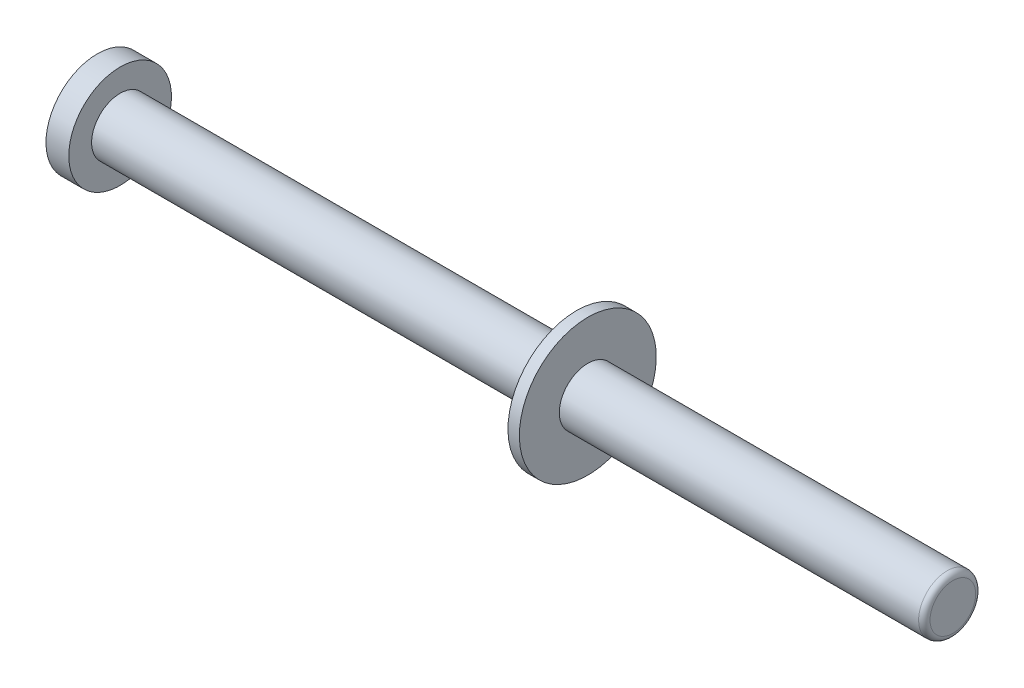
SolidWorks part; units mm, degrees
material "Plain Carbon Steel"
ref_plane "Front Plane" through (0, 0, 0) normal (0, 0, 1) x (1, 0, 0)
ref_plane "Top Plane" through (0, 0, 0) normal (0, 1, 0) x (1, 0, 0)
ref_plane "Right Plane" through (0, 0, 0) normal (1, 0, 0) x (0, 0, -1)
sketch "Shaft Profile Sketch" plane through (0, 0, 0) normal (0, 0, 1) x (1, 0, 0)
  line L0 (0, 0) -> (-150, 0) construction
  line L1 (-150, 0) -> (-150, 9)
  line L2 (-150, 9) -> (-146, 9)
  line L3 (-146, 9) -> (-146, 5)
  line L4 (-146, 5) -> (-66, 5)
  line L5 (-66, 5) -> (-66, 12)
  line L6 (-66, 12) -> (-64, 12)
  line L7 (-64, 12) -> (-64, 5)
  line L8 (-64, 5) -> (0, 5)
  line L9 (0, 5) -> (0, 0)
  line L10 (0, 0) -> (-150, 0)
  dimension "D1" = 9
  dimension "D2" = 5
  dimension "D3" = 12
  dimension "D4" = 2
  dimension "D5" = 4
  dimension "D6" = 80
  dimension "D7" = 64
revolve "Shaft Body Revolve" add sketch "Shaft Profile Sketch" angle 360 about L0
fillet "Edge Fillet R1" radius 1 1 edges at (0, 5, 0)
